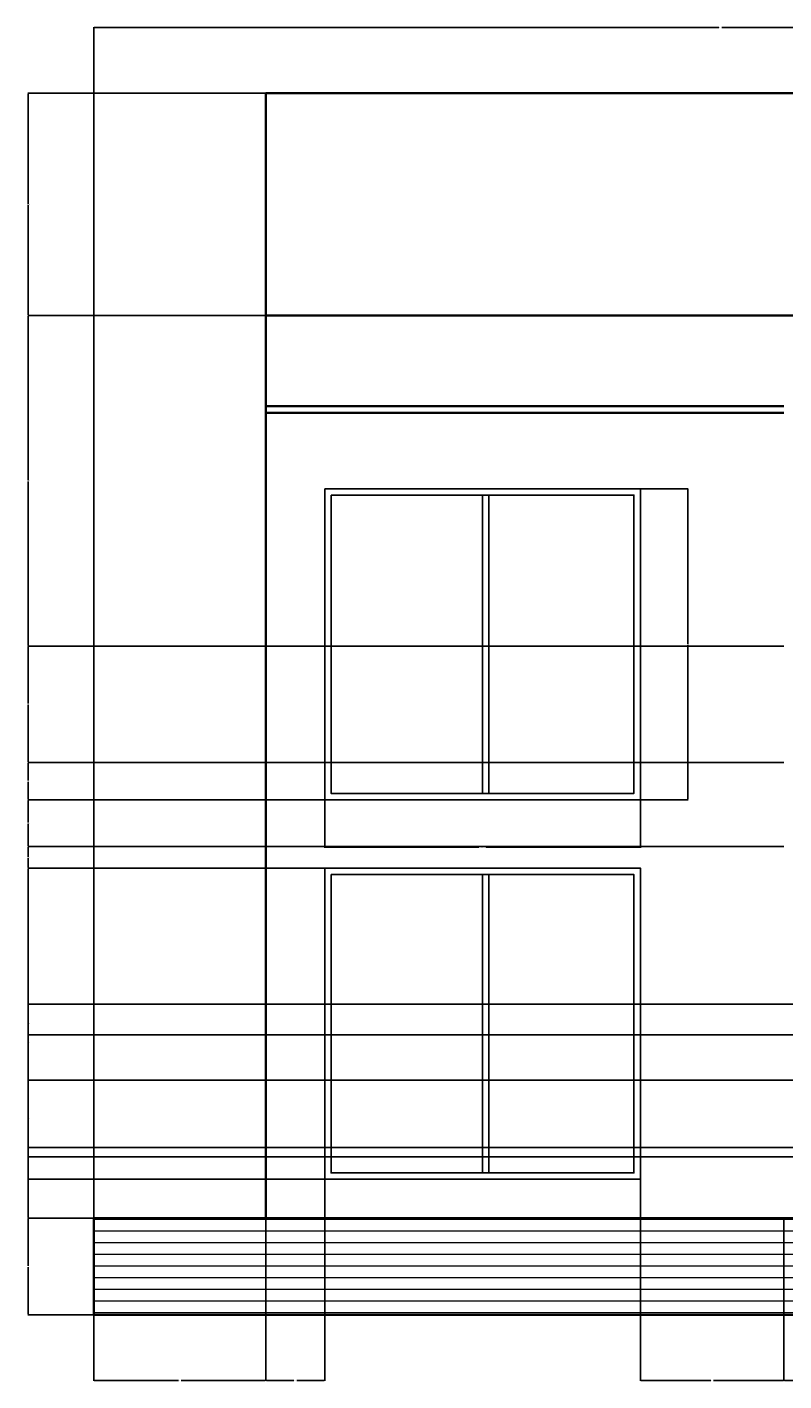
# Model space of a CAD drawing. Units: inches. Extents: x 18 to 448, y 19 to 438.
# Tile 1 of 2: x 18 to 253, y 19 to 438. Entities that reach past the tile are written whole.
import ezdxf

# ---------------------------------------------------------------- set-up
doc = ezdxf.new("R2010")
doc.units = ezdxf.units.IN
doc.header["$MEASUREMENT"] = 0
for name, color, linetype, lineweight in [('A-ANNO-DIMS', 2, 'Continuous', 18), ('A-ELEV', 7, 'Continuous', 35), ('A-ELEV-PATT', 8, 'Continuous', 13), ('A-GLAZ', 4, 'Continuous', 25)]:
    doc.layers.add(name, color=color, linetype=linetype, lineweight=lineweight)
doc.styles.get("Standard").update_dxf_attribs({"font": 'arial.ttf'})
doc.dimstyles.get("Standard").update_dxf_attribs({"dimtxt": 0.18, "dimasz": 0.18, "dimexe": 0.18, "dimexo": 0.0625, "dimgap": 0.09, "dimtad": 0, "dimtih": 1, "dimtoh": 1, "dimdec": 4, "dimzin": 0, "dimdsep": 46, "dimtxsty": 'Standard', "dimcen": 0.09, "dimadec": 0, "dimazin": 0, "dimtfac": 1, "dimtdec": 4, "dimtofl": 0, "dimtmove": 0, "dimatfit": 3, "dimfxl": 1, "dimtolj": 1, "dimtzin": 0, "dimarcsym": 0})

# ---------------------------------------------------------------- blocks, each defined once
blk = doc.blocks.new('WIN-1200x1200')
for p, q in [((49.42, 94.26), (49.42, 1.8)), ((51.42, 94.26), (51.42, 1.8))]:
    blk.add_line(p, q)
for points in [[(0.48, 96.26), (98.37, 96.26), (98.37, -0.2), (0.48, -0.2)], [(2.48, 94.26), (96.37, 94.26), (96.37, 1.8), (2.48, 1.8)]]:
    blk.add_lwpolyline(points, close=True)
blk = doc.blocks.new('*D3')
at = {"layer": 'A-ANNO-DIMS', "color": 0, "lineweight": -2, "transparency": 16777216}
for p, q in [((110.48, 198.73), (110.48, 183.93)), ((208.37, 198.73), (208.37, 183.93)), ((110.66, 184.11), (158.3, 184.11)), ((208.19, 184.11), (160.54, 184.11))]:
    blk.add_line(p, q, dxfattribs=at)
at = {"layer": 'A-ANNO-DIMS', "color": 0, "transparency": 16777216}
for points in [[(110.66, 184.14), (110.66, 184.08), (110.48, 184.11)], [(208.19, 184.14), (208.19, 184.08), (208.37, 184.11)]]:
    blk.add_solid(points, dxfattribs=at)
at = {"layer": 'Defpoints', "color": 0, "transparency": 16777216}
for p in [(110.48, 198.8), (208.37, 198.8), (208.37, 184.11)]:
    blk.add_point(p, dxfattribs=at)
at = {"layer": 'A-ANNO-DIMS', "color": 0, "transparency": 16777216, "insert": (159.42, 184.11), "char_height": 0.18, "attachment_point": 5}
blk.add_mtext('\\A1;WINDOW 98 TYP.', dxfattribs=at)
blk = doc.blocks.new('*D4')
at = {"layer": 'A-ANNO-DIMS', "color": 0, "lineweight": -2, "transparency": 16777216}
for p, q in [((208.43, 295.26), (223.23, 295.26)), ((223.05, 295.08), (223.05, 247.21)), ((223.05, 198.98), (223.05, 246.84)), ((208.43, 198.8), (223.23, 198.8))]:
    blk.add_line(p, q, dxfattribs=at)
at = {"layer": 'A-ANNO-DIMS', "color": 0, "transparency": 16777216}
for points in [[(223.02, 295.08), (223.08, 295.08), (223.05, 295.26)], [(223.02, 198.98), (223.08, 198.98), (223.05, 198.8)]]:
    blk.add_solid(points, dxfattribs=at)
at = {"layer": 'Defpoints', "color": 0, "transparency": 16777216}
for p in [(208.37, 295.26), (223.05, 295.26), (208.37, 198.8)]:
    blk.add_point(p, dxfattribs=at)
at = {"layer": 'A-ANNO-DIMS', "color": 0, "transparency": 16777216, "insert": (223.05, 247.03), "char_height": 0.18, "attachment_point": 5}
blk.add_mtext('\\A1;96 TYP.', dxfattribs=at)
blk = doc.blocks.new('*D7')
at = {"layer": 'A-ANNO-DIMS', "color": 0, "lineweight": -2, "transparency": 16777216}
for p, q in [((38.85, 39.26), (38.85, 438.34)), ((39.03, 438.16), (232.72, 438.16)), ((427.33, 438.16), (233.64, 438.16)), ((427.51, 39.26), (427.51, 438.34))]:
    blk.add_line(p, q, dxfattribs=at)
at = {"layer": 'A-ANNO-DIMS', "color": 0, "transparency": 16777216}
for points in [[(39.03, 438.19), (39.03, 438.13), (38.85, 438.16)], [(427.33, 438.19), (427.33, 438.13), (427.51, 438.16)]]:
    blk.add_solid(points, dxfattribs=at)
at = {"layer": 'Defpoints', "color": 0, "transparency": 16777216}
for p in [(427.51, 438.16), (38.85, 39.19), (427.51, 39.19)]:
    blk.add_point(p, dxfattribs=at)
at = {"layer": 'A-ANNO-DIMS', "color": 0, "transparency": 16777216, "insert": (233.18, 438.16), "char_height": 0.18, "attachment_point": 5}
blk.add_mtext('\\A1;388.66', dxfattribs=at)
blk = doc.blocks.new('*D9')
at = {"layer": 'A-ANNO-DIMS', "color": 0, "lineweight": -2, "transparency": 16777216}
for p, q in [((38.85, 69.13), (38.85, 18.71)), ((92.24, 69.13), (92.24, 18.71)), ((39.03, 18.89), (65.15, 18.89)), ((92.06, 18.89), (65.94, 18.89))]:
    blk.add_line(p, q, dxfattribs=at)
at = {"layer": 'A-ANNO-DIMS', "color": 0, "transparency": 16777216}
for points in [[(39.03, 18.92), (39.03, 18.86), (38.85, 18.89)], [(92.06, 18.92), (92.06, 18.86), (92.24, 18.89)]]:
    blk.add_solid(points, dxfattribs=at)
at = {"layer": 'Defpoints', "color": 0, "transparency": 16777216}
for p in [(38.85, 69.19), (92.24, 69.19), (92.24, 18.89)]:
    blk.add_point(p, dxfattribs=at)
at = {"layer": 'A-ANNO-DIMS', "color": 0, "transparency": 16777216, "insert": (65.55, 18.89), "char_height": 0.18, "attachment_point": 5}
blk.add_mtext('\\A1;53.39', dxfattribs=at)
blk = doc.blocks.new('*D10')
at = {"layer": 'A-ANNO-DIMS', "color": 0, "lineweight": -2, "transparency": 16777216}
for p, q in [((110.48, 81.14), (110.48, 18.71)), ((92.24, 69.13), (92.24, 18.71)), ((92.42, 18.89), (100.9, 18.89)), ((110.3, 18.89), (101.81, 18.89))]:
    blk.add_line(p, q, dxfattribs=at)
at = {"layer": 'A-ANNO-DIMS', "color": 0, "transparency": 16777216}
for points in [[(92.42, 18.92), (92.42, 18.86), (92.24, 18.89)], [(110.3, 18.92), (110.3, 18.86), (110.48, 18.89)]]:
    blk.add_solid(points, dxfattribs=at)
at = {"layer": 'Defpoints', "color": 0, "transparency": 16777216}
for p in [(110.48, 81.2), (92.24, 69.19), (110.48, 18.89)]:
    blk.add_point(p, dxfattribs=at)
at = {"layer": 'A-ANNO-DIMS', "color": 0, "transparency": 16777216, "insert": (101.36, 18.89), "char_height": 0.18, "attachment_point": 5}
blk.add_mtext('\\A1;18.234', dxfattribs=at)
blk = doc.blocks.new('*D11')
at = {"layer": 'A-ANNO-DIMS', "color": 0, "lineweight": -2, "transparency": 16777216}
for p, q in [((208.37, 81.14), (208.37, 18.71)), ((252.9, 69.13), (252.9, 18.71)), ((208.55, 18.89), (230.24, 18.89)), ((252.72, 18.89), (231.03, 18.89))]:
    blk.add_line(p, q, dxfattribs=at)
at = {"layer": 'A-ANNO-DIMS', "color": 0, "transparency": 16777216}
for points in [[(208.55, 18.92), (208.55, 18.86), (208.37, 18.89)], [(252.72, 18.92), (252.72, 18.86), (252.9, 18.89)]]:
    blk.add_solid(points, dxfattribs=at)
at = {"layer": 'Defpoints', "color": 0, "transparency": 16777216}
for p in [(208.37, 81.2), (252.9, 69.19), (252.9, 18.89)]:
    blk.add_point(p, dxfattribs=at)
at = {"layer": 'A-ANNO-DIMS', "color": 0, "transparency": 16777216, "insert": (230.64, 18.89), "char_height": 0.18, "attachment_point": 5}
blk.add_mtext('\\A1;44.54', dxfattribs=at)
blk = doc.blocks.new('*D12')
at = {"layer": 'A-ANNO-DIMS', "color": 0, "lineweight": -2, "transparency": 16777216}
for p, q in [((252.9, 69.13), (252.9, 18.71)), ((320.74, 69.13), (320.74, 18.71)), ((253.08, 18.89), (286.43, 18.89)), ((320.56, 18.89), (287.21, 18.89))]:
    blk.add_line(p, q, dxfattribs=at)
at = {"layer": 'A-ANNO-DIMS', "color": 0, "transparency": 16777216}
for points in [[(253.08, 18.92), (253.08, 18.86), (252.9, 18.89)], [(320.56, 18.92), (320.56, 18.86), (320.74, 18.89)]]:
    blk.add_solid(points, dxfattribs=at)
at = {"layer": 'Defpoints', "color": 0, "transparency": 16777216}
for p in [(252.9, 69.19), (320.74, 69.19), (320.74, 18.89)]:
    blk.add_point(p, dxfattribs=at)
at = {"layer": 'A-ANNO-DIMS', "color": 0, "transparency": 16777216, "insert": (286.82, 18.89), "char_height": 0.18, "attachment_point": 5}
blk.add_mtext('\\A1;67.83', dxfattribs=at)
blk = doc.blocks.new('*D15')
at = {"layer": 'A-ANNO-DIMS', "color": 0, "lineweight": -2, "transparency": 16777216}
for p, q in [((38.79, 69.19), (18.37, 69.19)), ((18.55, 69.01), (18.55, 54.38)), ((18.55, 39.37), (18.55, 54.01)), ((38.79, 39.19), (18.37, 39.19))]:
    blk.add_line(p, q, dxfattribs=at)
at = {"layer": 'A-ANNO-DIMS', "color": 0, "transparency": 16777216}
for points in [[(18.52, 69.01), (18.58, 69.01), (18.55, 69.19)], [(18.52, 39.37), (18.58, 39.37), (18.55, 39.19)]]:
    blk.add_solid(points, dxfattribs=at)
at = {"layer": 'Defpoints', "color": 0, "transparency": 16777216}
for p in [(18.55, 69.19), (38.85, 69.19), (38.85, 39.19)]:
    blk.add_point(p, dxfattribs=at)
at = {"layer": 'A-ANNO-DIMS', "color": 0, "transparency": 16777216, "insert": (18.55, 54.19), "char_height": 0.18, "attachment_point": 5}
blk.add_mtext('\\A1;30', dxfattribs=at)
blk = doc.blocks.new('*D16')
at = {"layer": 'A-ANNO-DIMS', "color": 0, "lineweight": -2, "transparency": 16777216}
for p, q in [((110.41, 81.2), (18.37, 81.2)), ((18.55, 81.02), (18.55, 75.38)), ((18.55, 69.37), (18.55, 75.02)), ((92.18, 69.19), (18.37, 69.19))]:
    blk.add_line(p, q, dxfattribs=at)
at = {"layer": 'A-ANNO-DIMS', "color": 0, "transparency": 16777216}
for points in [[(18.52, 81.02), (18.58, 81.02), (18.55, 81.2)], [(18.52, 69.37), (18.58, 69.37), (18.55, 69.19)]]:
    blk.add_solid(points, dxfattribs=at)
at = {"layer": 'Defpoints', "color": 0, "transparency": 16777216}
for p in [(18.55, 81.2), (110.48, 81.2), (92.24, 69.19)]:
    blk.add_point(p, dxfattribs=at)
at = {"layer": 'A-ANNO-DIMS', "color": 0, "transparency": 16777216, "insert": (18.55, 75.2), "char_height": 0.18, "attachment_point": 5}
blk.add_mtext('\\A1;12.01', dxfattribs=at)
blk = doc.blocks.new('*D17')
at = {"layer": 'A-ANNO-DIMS', "color": 0, "lineweight": -2, "transparency": 16777216}
for p, q in [((110.41, 177.66), (18.37, 177.66)), ((18.55, 177.48), (18.55, 129.62)), ((18.55, 81.38), (18.55, 129.25)), ((110.41, 81.2), (18.37, 81.2))]:
    blk.add_line(p, q, dxfattribs=at)
at = {"layer": 'A-ANNO-DIMS', "color": 0, "transparency": 16777216}
for points in [[(18.52, 177.48), (18.58, 177.48), (18.55, 177.66)], [(18.52, 81.38), (18.58, 81.38), (18.55, 81.2)]]:
    blk.add_solid(points, dxfattribs=at)
at = {"layer": 'Defpoints', "color": 0, "transparency": 16777216}
for p in [(18.55, 177.66), (110.48, 177.66), (110.48, 81.2)]:
    blk.add_point(p, dxfattribs=at)
at = {"layer": 'A-ANNO-DIMS', "color": 0, "transparency": 16777216, "insert": (18.55, 129.43), "char_height": 0.18, "attachment_point": 5}
blk.add_mtext('\\A1;96.46', dxfattribs=at)
blk = doc.blocks.new('*D18')
at = {"layer": 'A-ANNO-DIMS', "color": 0, "lineweight": -2, "transparency": 16777216}
for p, q in [((252.84, 184.34), (18.37, 184.34)), ((18.55, 184.16), (18.55, 181.19)), ((18.55, 177.84), (18.55, 180.82)), ((110.41, 177.66), (18.37, 177.66))]:
    blk.add_line(p, q, dxfattribs=at)
at = {"layer": 'A-ANNO-DIMS', "color": 0, "transparency": 16777216}
for points in [[(18.52, 184.16), (18.58, 184.16), (18.55, 184.34)], [(18.52, 177.84), (18.58, 177.84), (18.55, 177.66)]]:
    blk.add_solid(points, dxfattribs=at)
at = {"layer": 'Defpoints', "color": 0, "transparency": 16777216}
for p in [(18.55, 184.34), (252.9, 184.34), (110.48, 177.66)]:
    blk.add_point(p, dxfattribs=at)
at = {"layer": 'A-ANNO-DIMS', "color": 0, "transparency": 16777216, "insert": (18.55, 181), "char_height": 0.18, "attachment_point": 5}
blk.add_mtext('\\A1;6.679', dxfattribs=at)
blk = doc.blocks.new('*D19')
at = {"layer": 'A-ANNO-DIMS', "color": 0, "lineweight": -2, "transparency": 16777216}
for p, q in [((110.41, 198.8), (18.37, 198.8)), ((18.55, 198.62), (18.55, 191.75)), ((18.55, 184.52), (18.55, 191.39)), ((252.84, 184.34), (18.37, 184.34))]:
    blk.add_line(p, q, dxfattribs=at)
at = {"layer": 'A-ANNO-DIMS', "color": 0, "transparency": 16777216}
for points in [[(18.52, 198.62), (18.58, 198.62), (18.55, 198.8)], [(18.52, 184.52), (18.58, 184.52), (18.55, 184.34)]]:
    blk.add_solid(points, dxfattribs=at)
at = {"layer": 'Defpoints', "color": 0, "transparency": 16777216}
for p in [(18.55, 198.8), (110.48, 198.8), (252.9, 184.34)]:
    blk.add_point(p, dxfattribs=at)
at = {"layer": 'A-ANNO-DIMS', "color": 0, "transparency": 16777216, "insert": (18.55, 191.57), "char_height": 0.18, "attachment_point": 5}
blk.add_mtext('\\A1;14.452', dxfattribs=at)
blk = doc.blocks.new('*D20')
at = {"layer": 'A-ANNO-DIMS', "color": 0, "lineweight": -2, "transparency": 16777216}
for p, q in [((252.84, 210.4), (18.37, 210.4)), ((18.55, 210.22), (18.55, 204.78)), ((18.55, 198.98), (18.55, 204.42)), ((110.41, 198.8), (18.37, 198.8))]:
    blk.add_line(p, q, dxfattribs=at)
at = {"layer": 'A-ANNO-DIMS', "color": 0, "transparency": 16777216}
for points in [[(18.52, 210.22), (18.58, 210.22), (18.55, 210.4)], [(18.52, 198.98), (18.58, 198.98), (18.55, 198.8)]]:
    blk.add_solid(points, dxfattribs=at)
at = {"layer": 'Defpoints', "color": 0, "transparency": 16777216}
for p in [(18.55, 210.4), (252.9, 210.4), (110.48, 198.8)]:
    blk.add_point(p, dxfattribs=at)
at = {"layer": 'A-ANNO-DIMS', "color": 0, "transparency": 16777216, "insert": (18.55, 204.6), "char_height": 0.18, "attachment_point": 5}
blk.add_mtext('\\A1;11.609', dxfattribs=at)
blk = doc.blocks.new('*D21')
at = {"layer": 'A-ANNO-DIMS', "color": 0, "lineweight": -2, "transparency": 16777216}
for p, q in [((252.84, 246.49), (18.37, 246.49)), ((18.55, 246.31), (18.55, 228.63)), ((18.55, 210.58), (18.55, 228.27)), ((252.84, 210.4), (18.37, 210.4))]:
    blk.add_line(p, q, dxfattribs=at)
at = {"layer": 'A-ANNO-DIMS', "color": 0, "transparency": 16777216}
for points in [[(18.52, 246.31), (18.58, 246.31), (18.55, 246.49)], [(18.52, 210.58), (18.58, 210.58), (18.55, 210.4)]]:
    blk.add_solid(points, dxfattribs=at)
at = {"layer": 'Defpoints', "color": 0, "transparency": 16777216}
for p in [(18.55, 246.49), (252.9, 246.49), (252.9, 210.4)]:
    blk.add_point(p, dxfattribs=at)
at = {"layer": 'A-ANNO-DIMS', "color": 0, "transparency": 16777216, "insert": (18.55, 228.45), "char_height": 0.18, "attachment_point": 5}
blk.add_mtext('\\A1;36.086', dxfattribs=at)
blk = doc.blocks.new('*D22')
at = {"layer": 'A-ANNO-DIMS', "color": 0, "lineweight": -2, "transparency": 16777216}
for p, q in [((92.18, 348.92), (18.37, 348.92)), ((18.55, 348.74), (18.55, 297.89)), ((18.55, 246.67), (18.55, 297.53)), ((252.84, 246.49), (18.37, 246.49))]:
    blk.add_line(p, q, dxfattribs=at)
at = {"layer": 'A-ANNO-DIMS', "color": 0, "transparency": 16777216}
for points in [[(18.52, 348.74), (18.58, 348.74), (18.55, 348.92)], [(18.52, 246.67), (18.58, 246.67), (18.55, 246.49)]]:
    blk.add_solid(points, dxfattribs=at)
at = {"layer": 'Defpoints', "color": 0, "transparency": 16777216}
for p in [(18.55, 348.92), (92.24, 348.92), (252.9, 246.49)]:
    blk.add_point(p, dxfattribs=at)
at = {"layer": 'A-ANNO-DIMS', "color": 0, "transparency": 16777216, "insert": (18.55, 297.71), "char_height": 0.18, "attachment_point": 5}
blk.add_mtext('\\A1;102.43', dxfattribs=at)
blk = doc.blocks.new('*D23')
at = {"layer": 'A-ANNO-DIMS', "color": 0, "lineweight": -2, "transparency": 16777216}
for p, q in [((92.18, 417.86), (18.37, 417.86)), ((18.55, 417.68), (18.55, 383.57)), ((18.55, 349.1), (18.55, 383.21)), ((92.18, 348.92), (18.37, 348.92))]:
    blk.add_line(p, q, dxfattribs=at)
at = {"layer": 'A-ANNO-DIMS', "color": 0, "transparency": 16777216}
for points in [[(18.52, 417.68), (18.58, 417.68), (18.55, 417.86)], [(18.52, 349.1), (18.58, 349.1), (18.55, 348.92)]]:
    blk.add_solid(points, dxfattribs=at)
at = {"layer": 'Defpoints', "color": 0, "transparency": 16777216}
for p in [(18.55, 417.86), (92.24, 417.86), (92.24, 348.92)]:
    blk.add_point(p, dxfattribs=at)
at = {"layer": 'A-ANNO-DIMS', "color": 0, "transparency": 16777216, "insert": (18.55, 383.39), "char_height": 0.18, "attachment_point": 5}
blk.add_mtext('\\A1;68.93', dxfattribs=at)
blk = doc.blocks.new('*D42')
at = {"layer": 'A-ANNO-DIMS', "color": 0, "lineweight": -2, "transparency": 16777216}
for p, q in [((345.81, 111.98), (18.37, 111.98)), ((18.55, 111.8), (18.55, 100.23)), ((18.55, 88.31), (18.55, 99.87)), ((345.81, 88.13), (18.37, 88.13))]:
    blk.add_line(p, q, dxfattribs=at)
at = {"layer": 'A-ANNO-DIMS', "color": 0, "transparency": 16777216}
for points in [[(18.52, 111.8), (18.58, 111.8), (18.55, 111.98)], [(18.52, 88.31), (18.58, 88.31), (18.55, 88.13)]]:
    blk.add_solid(points, dxfattribs=at)
at = {"layer": 'Defpoints', "color": 0, "transparency": 16777216}
for p in [(18.55, 111.98), (345.87, 111.98), (345.87, 88.13)]:
    blk.add_point(p, dxfattribs=at)
at = {"layer": 'A-ANNO-DIMS', "color": 0, "transparency": 16777216, "insert": (18.55, 100.05), "char_height": 0.18, "attachment_point": 5}
blk.add_mtext('\\A1;23.85', dxfattribs=at)
blk = doc.blocks.new('*D43')
at = {"layer": 'A-ANNO-DIMS', "color": 0, "lineweight": -2, "transparency": 16777216}
for p, q in [((345.81, 135.54), (18.37, 135.54)), ((18.55, 135.36), (18.55, 123.94)), ((18.55, 112.16), (18.55, 123.58)), ((345.81, 111.98), (18.37, 111.98))]:
    blk.add_line(p, q, dxfattribs=at)
at = {"layer": 'A-ANNO-DIMS', "color": 0, "transparency": 16777216}
for points in [[(18.52, 135.36), (18.58, 135.36), (18.55, 135.54)], [(18.52, 112.16), (18.58, 112.16), (18.55, 111.98)]]:
    blk.add_solid(points, dxfattribs=at)
at = {"layer": 'Defpoints', "color": 0, "transparency": 16777216}
for p in [(18.55, 135.54), (345.87, 135.54), (345.87, 111.98)]:
    blk.add_point(p, dxfattribs=at)
at = {"layer": 'A-ANNO-DIMS', "color": 0, "transparency": 16777216, "insert": (18.55, 123.76), "char_height": 0.18, "attachment_point": 5}
blk.add_mtext('\\A1;23.56', dxfattribs=at)
blk = doc.blocks.new('*D44')
at = {"layer": 'A-ANNO-DIMS', "color": 0, "lineweight": -2, "transparency": 16777216}
for p, q in [((391.16, 91.09), (18.37, 91.09)), ((18.55, 90.91), (18.55, 80.33)), ((18.55, 69.37), (18.55, 79.96)), ((373.54, 69.19), (18.37, 69.19))]:
    blk.add_line(p, q, dxfattribs=at)
at = {"layer": 'A-ANNO-DIMS', "color": 0, "transparency": 16777216}
for points in [[(18.52, 90.91), (18.58, 90.91), (18.55, 91.09)], [(18.52, 69.37), (18.58, 69.37), (18.55, 69.19)]]:
    blk.add_solid(points, dxfattribs=at)
at = {"layer": 'Defpoints', "color": 0, "transparency": 16777216}
for p in [(18.55, 91.09), (391.23, 91.09), (373.61, 69.19)]:
    blk.add_point(p, dxfattribs=at)
at = {"layer": 'A-ANNO-DIMS', "color": 0, "transparency": 16777216, "insert": (18.55, 80.14), "char_height": 0.18, "attachment_point": 5}
blk.add_mtext('\\A1;21.9', dxfattribs=at)
blk = doc.blocks.new('*D45')
at = {"layer": 'A-ANNO-DIMS', "color": 0, "lineweight": -2, "transparency": 16777216}
for p, q in [((391.16, 125.99), (18.37, 125.99)), ((18.55, 125.81), (18.55, 108.73)), ((18.55, 91.27), (18.55, 108.36)), ((391.16, 91.09), (18.37, 91.09))]:
    blk.add_line(p, q, dxfattribs=at)
at = {"layer": 'A-ANNO-DIMS', "color": 0, "transparency": 16777216}
for points in [[(18.52, 125.81), (18.58, 125.81), (18.55, 125.99)], [(18.52, 91.27), (18.58, 91.27), (18.55, 91.09)]]:
    blk.add_solid(points, dxfattribs=at)
at = {"layer": 'Defpoints', "color": 0, "transparency": 16777216}
for p in [(18.55, 125.99), (391.23, 125.99), (391.23, 91.09)]:
    blk.add_point(p, dxfattribs=at)
at = {"layer": 'A-ANNO-DIMS', "color": 0, "transparency": 16777216, "insert": (18.55, 108.54), "char_height": 0.18, "attachment_point": 5}
blk.add_mtext('\\A1;34.9', dxfattribs=at)

msp = doc.modelspace()

# ---------------------------------------------------------------- hatches: boundary and pattern name
at = {"layer": 'A-ELEV-PATT'}
h = msp.add_hatch(dxfattribs=at)
h.set_pattern_fill('ANSI31', color=256, scale=29, angle=135)
h.paths.add_polyline_path([(320.7354, 59.1939), (320.7354, 69.1939), (38.8517, 69.1939), (38.8517, 39.1939), (320.7354, 39.1939), (320.7354, 49.1939)])

# ---------------------------------------------------------------- linework, layer by layer
at = {"layer": 'A-ELEV'}
for p, q in [((92.2414, 348.9241), (92.2414, 417.8553)), ((92.2414, 417.8553), (320.7354, 417.8553)), ((92.2414, 318.796), (92.2414, 348.9241)), ((92.2414, 348.9241), (427.508, 348.9241)), ((92.2414, 320.796), (252.9033, 320.796)), ((92.2414, 198.796), (92.2414, 318.796)), ((92.2414, 318.796), (252.9033, 318.796)), ((92.2414, 69.1939), (92.2414, 198.796)), ((38.8517, 69.1939), (427.508, 69.1939)), ((38.8517, 39.1939), (38.8517, 69.1939)), ((320.7354, 39.1939), (38.8517, 39.1939))]:
    msp.add_line(p, q, dxfattribs=at)

# ---------------------------------------------------------------- block references
at = {"layer": 'A-GLAZ'}
for p in [(110, 199), (110, 81.4069)]:
    msp.add_blockref('WIN-1200x1200', p, dxfattribs=at)

# ---------------------------------------------------------------- dimensions: what is measured, and where the dimension line sits
at = {"layer": 'A-ANNO-DIMS'}
for base, p1, p2, override, picture, middle in [((427.508, 438.1553), (38.8517, 39.1939), (427.508, 39.1939), {"dimdec": 2, "dimlfac": 1, "dimrnd": 0, "dimzin": 0, "dimdsep": 46, "dimlunit": 2}, '*D7', (233.1799, 438.1553)), ((110.4754, 18.8939), (92.2414, 69.1939), (110.4754, 81.2029), {"dimdec": 3, "dimlfac": 1, "dimrnd": 0, "dimzin": 0, "dimdsep": 46, "dimlunit": 2}, '*D10', (101.3584, 18.8939)), ((252.9033, 18.8939), (208.3671, 81.2029), (252.9033, 69.1939), {"dimdec": 2, "dimlfac": 1, "dimrnd": 0, "dimzin": 0, "dimdsep": 46, "dimlunit": 2}, '*D11', (230.6352, 18.8939)), ((92.2414, 18.8939), (38.8517, 69.1939), (92.2414, 69.1939), {"dimdec": 2, "dimlfac": 1, "dimrnd": 0, "dimzin": 0, "dimdsep": 46, "dimlunit": 2}, '*D9', (65.5466, 18.8939)), ((320.7354, 18.8939), (252.9033, 69.1939), (320.7354, 69.1939), {"dimdec": 2, "dimlfac": 1, "dimrnd": 0, "dimzin": 0, "dimdsep": 46, "dimlunit": 2}, '*D12', (286.8193, 18.8939))]:
    dim = msp.add_linear_dim(base=base, p1=p1, p2=p2, dimstyle='Standard', override=override, dxfattribs=at)
    dim.commit()
    dim.dimension.update_dxf_attribs({"geometry": picture, "text_midpoint": middle})
for base, p1, p2, override, picture, middle in [((18.5517, 417.8553), (92.2414, 348.9241), (92.2414, 417.8553), {"dimdec": 2, "dimlfac": 1, "dimrnd": 0, "dimzin": 0, "dimdsep": 46, "dimlunit": 2}, '*D23', (18.5517, 383.3897)), ((18.5517, 348.9241), (252.9033, 246.4909), (92.2414, 348.9241), {"dimdec": 2, "dimlfac": 1, "dimrnd": 0, "dimzin": 0, "dimdsep": 46, "dimlunit": 2}, '*D22', (18.5517, 297.7075)), ((18.5517, 246.4909), (252.9033, 210.4047), (252.9033, 246.4909), {"dimdec": 3, "dimlfac": 1, "dimrnd": 0, "dimzin": 0, "dimdsep": 46, "dimlunit": 2}, '*D21', (18.5517, 228.4478)), ((18.5517, 210.4047), (110.4754, 198.796), (252.9033, 210.4047), {"dimdec": 3, "dimlfac": 1, "dimrnd": 0, "dimzin": 0, "dimdsep": 46, "dimlunit": 2}, '*D20', (18.5517, 204.6003)), ((18.5517, 198.796), (252.9033, 184.3438), (110.4754, 198.796), {"dimdec": 3, "dimlfac": 1, "dimrnd": 0, "dimzin": 0, "dimdsep": 46, "dimlunit": 2}, '*D19', (18.5517, 191.5699)), ((18.5517, 184.3438), (110.4754, 177.6645), (252.9033, 184.3438), {"dimdec": 3, "dimlfac": 1, "dimrnd": 0, "dimzin": 0, "dimdsep": 46, "dimlunit": 2}, '*D18', (18.5517, 181.0042)), ((18.5517, 177.6645), (110.4754, 81.2029), (110.4754, 177.6645), {"dimdec": 2, "dimlfac": 1, "dimrnd": 0, "dimzin": 0, "dimdsep": 46, "dimlunit": 2}, '*D17', (18.5517, 129.4337)), ((18.5517, 135.5385), (345.8731, 111.9775), (345.8731, 135.5385), {"dimdec": 2, "dimlfac": 1, "dimrnd": 0, "dimzin": 0, "dimdsep": 46, "dimlunit": 2}, '*D43', (18.5517, 123.758)), ((18.5517, 125.9945), (391.2265, 91.0931), (391.2265, 125.9945), {"dimdec": 1, "dimlfac": 1, "dimrnd": 0, "dimzin": 0, "dimdsep": 46, "dimlunit": 2}, '*D45', (18.5517, 108.5438)), ((18.5517, 111.9775), (345.8731, 88.1277), (345.8731, 111.9775), {"dimdec": 2, "dimlfac": 1, "dimrnd": 0, "dimzin": 0, "dimdsep": 46, "dimlunit": 2}, '*D42', (18.5517, 100.0526)), ((18.5517, 91.0931), (373.6066, 69.1939), (391.2265, 91.0931), {"dimdec": 1, "dimlfac": 1, "dimrnd": 0, "dimzin": 0, "dimdsep": 46, "dimlunit": 2}, '*D44', (18.5517, 80.1435)), ((18.5517, 81.2029), (92.2414, 69.1939), (110.4754, 81.2029), {"dimdec": 2, "dimlfac": 1, "dimrnd": 0, "dimzin": 0, "dimdsep": 46, "dimlunit": 2}, '*D16', (18.5517, 75.1984)), ((18.5517, 69.1939), (38.8517, 39.1939), (38.8517, 69.1939), {"dimdec": 0, "dimlfac": 1, "dimrnd": 0, "dimzin": 0, "dimdsep": 46, "dimlunit": 2}, '*D15', (18.5517, 54.1939))]:
    dim = msp.add_linear_dim(base=base, p1=p1, p2=p2, angle=90, dimstyle='Standard', override=override, dxfattribs=at)
    dim.commit()
    dim.dimension.update_dxf_attribs({"geometry": picture, "text_midpoint": middle})
dim = msp.add_linear_dim(base=(223.0509, 295.2577), p1=(208.3671, 198.796), p2=(208.3671, 295.2577), angle=90, text='<> TYP.', dimstyle='Standard', override={"dimdec": 0, "dimlfac": 1, "dimrnd": 0, "dimzin": 0, "dimdsep": 46, "dimlunit": 2}, dxfattribs=at)
dim.commit()
dim.dimension.update_dxf_attribs({"geometry": '*D4', "text_midpoint": (223.0509, 247.0269)})
dim = msp.add_linear_dim(base=(208.3671, 184.1123), p1=(110.4754, 198.796), p2=(208.3671, 198.796), text='WINDOW <> TYP.', dimstyle='Standard', override={"dimdec": 0, "dimlfac": 1, "dimrnd": 0, "dimzin": 0, "dimdsep": 46, "dimlunit": 2}, dxfattribs=at)
dim.commit()
dim.dimension.update_dxf_attribs({"geometry": '*D3', "text_midpoint": (159.4213, 184.1123)})

doc.saveas('drawing.dxf')
